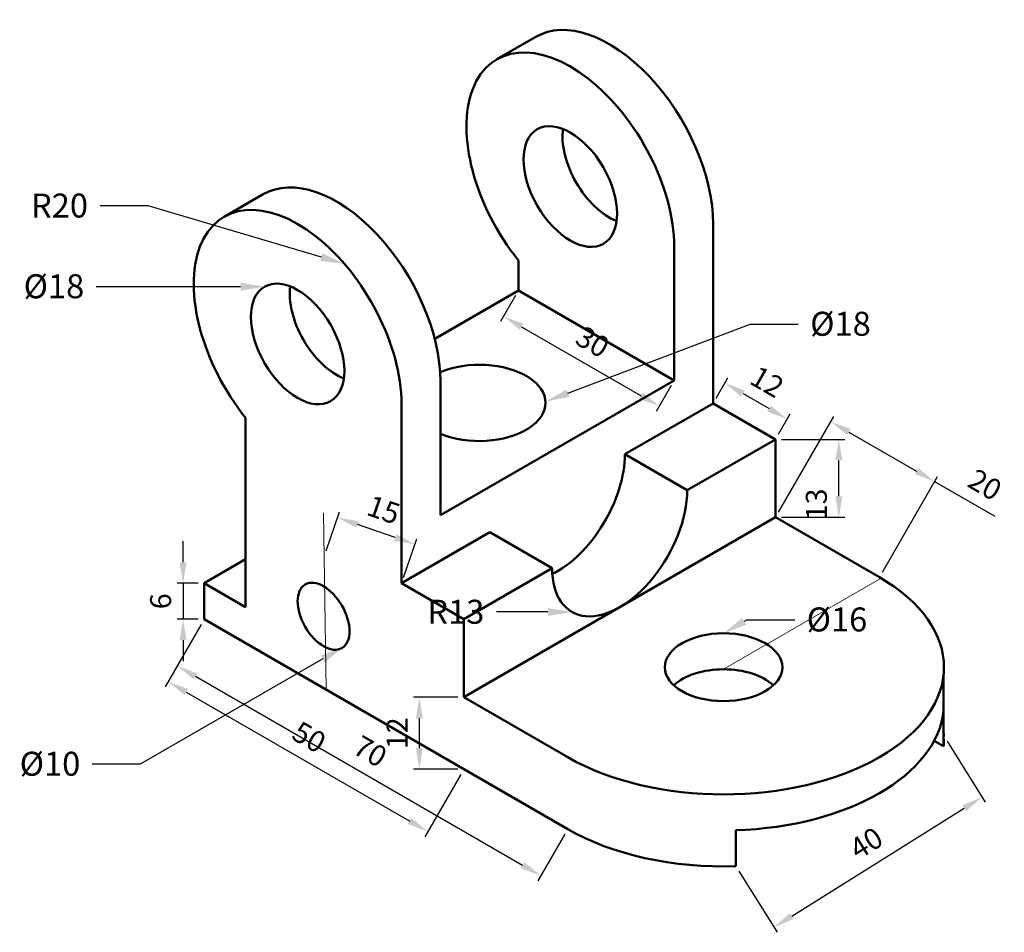
# Model space of a CAD drawing. Units: millimetres. Extents: x 1541 to 1705, y 1721 to 1873.
import ezdxf
from ezdxf import colors
from ezdxf.entities.mleader import LeaderData, LeaderLine
from ezdxf.math import Vec2, Vec3

# ---------------------------------------------------------------- set-up
doc = ezdxf.new("R2010")
doc.units = ezdxf.units.MM
doc.linetypes.add('CENTER', pattern=[50.8, 31.75, -6.35, 6.35, -6.35])
for name, color, linetype, lineweight in [('M-CNTR', 4, 'CENTER', 18), ('M-DIMS', 3, 'Continuous', 25), ('M-OUTL', 7, 'Continuous', 50)]:
    doc.layers.add(name, color=color, linetype=linetype, lineweight=lineweight)
doc.styles.get("Standard").update_dxf_attribs({"font": 'arial.ttf'})
doc.dimstyles.new('AM_ISO$0', dxfattribs={"dimtxt": 3.5, "dimasz": 3.5, "dimexe": 1, "dimexo": 1, "dimgap": 1.5, "dimtad": 1, "dimdsep": 46, "dimtxsty": 'Standard', "dimcen": 0, "dimclrd": 256, "dimclre": 256, "dimclrt": 2, "dimadec": 0, "dimazin": 2, "dimtp": 0.1, "dimtm": 0.1, "dimtfac": 0.71, "dimtdec": 3, "dimtmove": 0, "dimatfit": 3, "dimfxl": 1, "dimlwd": -1, "dimlwe": -1, "dimarcsym": 1})

# ---------------------------------------------------------------- blocks, each defined once
blk = doc.blocks.new('*D3')
at = {"layer": 'Defpoints', "color": 0, "transparency": 16777216}
for p in [(1656.46, 1808.91), (1668.8, 1806.29), (1666.85, 1802.91)]:
    blk.add_point(p, dxfattribs=at)
at = {"layer": 'M-DIMS', "color": 0, "linetype": 'ByBlock', "transparency": 16777216}
for p, q in [((1656.96, 1809.78), (1658.91, 1813.16)), ((1661.44, 1810.54), (1665.77, 1808.04)), ((1667.35, 1803.78), (1669.3, 1807.16))]:
    blk.add_line(p, q, dxfattribs=at)
at = {"layer": 'M-DIMS', "color": 0, "transparency": 16777216}
for points in [[(1661.73, 1811.05), (1661.15, 1810.04), (1658.41, 1812.29)], [(1666.06, 1808.55), (1665.48, 1807.54), (1668.8, 1806.29)]]:
    blk.add_solid(points, dxfattribs=at)
at = {"layer": 'M-DIMS', "color": 0, "transparency": 16777216, "insert": (1665.23, 1812.12), "char_height": 3.5, "attachment_point": 5, "rotation": 330}
blk.add_mtext('12', dxfattribs=at)
blk = doc.blocks.new('*D4')
at = {"layer": 'Defpoints', "color": 0, "transparency": 16777216}
for p in [(1571.59, 1778.91), (1568.08, 1772.91), (1571.59, 1772.91)]:
    blk.add_point(p, dxfattribs=at)
at = {"layer": 'M-DIMS', "color": 0, "linetype": 'ByBlock', "transparency": 16777216}
for p, q in [((1568.08, 1782.41), (1568.08, 1785.91)), ((1570.59, 1778.91), (1567.08, 1778.91)), ((1568.08, 1778.91), (1568.08, 1772.91)), ((1570.59, 1772.91), (1567.08, 1772.91)), ((1568.08, 1769.41), (1568.08, 1765.91))]:
    blk.add_line(p, q, dxfattribs=at)
at = {"layer": 'M-DIMS', "color": 0, "transparency": 16777216}
for points in [[(1567.5, 1782.41), (1568.66, 1782.41), (1568.08, 1778.91)], [(1567.5, 1769.41), (1568.66, 1769.41), (1568.08, 1772.91)]]:
    blk.add_solid(points, dxfattribs=at)
at = {"layer": 'M-DIMS', "color": 0, "transparency": 16777216, "insert": (1564.79, 1775.91), "char_height": 3.5, "attachment_point": 5, "rotation": 90}
blk.add_mtext('6', dxfattribs=at)
blk = doc.blocks.new('*D5')
at = {"layer": 'Defpoints', "color": 0, "transparency": 16777216}
for p in [(1607.47, 1759.91), (1614.89, 1759.91), (1614.89, 1747.91)]:
    blk.add_point(p, dxfattribs=at)
at = {"layer": 'M-DIMS', "color": 0, "linetype": 'ByBlock', "transparency": 16777216}
for p, q in [((1613.89, 1759.91), (1606.47, 1759.91)), ((1607.47, 1751.41), (1607.47, 1756.41)), ((1613.89, 1747.91), (1606.47, 1747.91))]:
    blk.add_line(p, q, dxfattribs=at)
at = {"layer": 'M-DIMS', "color": 0, "transparency": 16777216}
for points in [[(1606.89, 1756.41), (1608.06, 1756.41), (1607.47, 1759.91)], [(1606.89, 1751.41), (1608.06, 1751.41), (1607.47, 1747.91)]]:
    blk.add_solid(points, dxfattribs=at)
at = {"layer": 'M-DIMS', "color": 0, "transparency": 16777216, "insert": (1604.21, 1753.91), "char_height": 3.5, "attachment_point": 5, "rotation": 90}
blk.add_mtext('12', dxfattribs=at)
blk = doc.blocks.new('*D6')
at = {"layer": 'Defpoints', "color": 0, "transparency": 16777216}
for p in [(1694.92, 1753.43), (1701.28, 1743.26), (1660.23, 1731.73)]:
    blk.add_point(p, dxfattribs=at)
at = {"layer": 'M-DIMS', "color": 0, "linetype": 'ByBlock', "transparency": 16777216}
for p, q in [((1695.45, 1752.58), (1701.81, 1742.41)), ((1669.56, 1723.42), (1698.32, 1741.4)), ((1660.76, 1730.89), (1667.13, 1720.71))]:
    blk.add_line(p, q, dxfattribs=at)
at = {"layer": 'M-DIMS', "color": 0, "transparency": 16777216}
for points in [[(1698.01, 1741.9), (1698.63, 1740.91), (1701.28, 1743.26)], [(1669.25, 1723.91), (1669.87, 1722.92), (1666.6, 1721.56)]]:
    blk.add_solid(points, dxfattribs=at)
at = {"layer": 'M-DIMS', "color": 0, "transparency": 16777216, "insert": (1682.2, 1735.2), "char_height": 3.5, "attachment_point": 5, "rotation": 32.027}
blk.add_mtext('40', dxfattribs=at)
blk = doc.blocks.new('*D7')
at = {"layer": 'Defpoints', "color": 0, "transparency": 16777216}
for p in [(1666.85, 1802.91), (1677.4, 1802.91), (1666.85, 1789.91)]:
    blk.add_point(p, dxfattribs=at)
at = {"layer": 'M-DIMS', "color": 0, "linetype": 'ByBlock', "transparency": 16777216}
for p, q in [((1667.85, 1802.91), (1678.4, 1802.91)), ((1677.4, 1793.41), (1677.4, 1799.41)), ((1667.85, 1789.91), (1678.4, 1789.91))]:
    blk.add_line(p, q, dxfattribs=at)
at = {"layer": 'M-DIMS', "color": 0, "transparency": 16777216}
for points in [[(1676.82, 1799.41), (1677.99, 1799.41), (1677.4, 1802.91)], [(1676.82, 1793.41), (1677.99, 1793.41), (1677.4, 1789.91)]]:
    blk.add_solid(points, dxfattribs=at)
at = {"layer": 'M-DIMS', "color": 0, "transparency": 16777216, "insert": (1674.11, 1792.06), "char_height": 3.5, "attachment_point": 5, "rotation": 90}
blk.add_mtext('13', dxfattribs=at)
blk = doc.blocks.new('*D8')
at = {"layer": 'Defpoints', "color": 0, "transparency": 16777216}
for p in [(1693.38, 1795.87), (1666.85, 1789.91), (1684.17, 1779.91)]:
    blk.add_point(p, dxfattribs=at)
at = {"layer": 'M-DIMS', "color": 0, "linetype": 'ByBlock', "transparency": 16777216}
for p, q in [((1667.35, 1790.78), (1676.56, 1806.74)), ((1679.09, 1804.12), (1690.35, 1797.62)), ((1684.67, 1780.78), (1693.88, 1796.74)), ((1693.38, 1795.87), (1703.4, 1790.09))]:
    blk.add_line(p, q, dxfattribs=at)
at = {"layer": 'M-DIMS', "color": 0, "transparency": 16777216}
for points in [[(1679.39, 1804.63), (1678.8, 1803.62), (1676.06, 1805.87)], [(1690.64, 1798.13), (1690.06, 1797.12), (1693.38, 1795.87)]]:
    blk.add_solid(points, dxfattribs=at)
at = {"layer": 'M-DIMS', "color": 0, "transparency": 16777216, "insert": (1701.55, 1794.96), "char_height": 3.5, "attachment_point": 5, "rotation": 330}
blk.add_mtext('20', dxfattribs=at)
blk = doc.blocks.new('*D9')
at = {"layer": 'Defpoints', "color": 0, "transparency": 16777216}
for p in [(1571.59, 1772.91), (1614.89, 1747.91), (1608.89, 1737.52)]:
    blk.add_point(p, dxfattribs=at)
at = {"layer": 'M-DIMS', "color": 0, "linetype": 'ByBlock', "transparency": 16777216}
for p, q in [((1571.09, 1772.05), (1565.09, 1761.66)), ((1568.62, 1760.77), (1605.86, 1739.27)), ((1614.39, 1747.05), (1608.39, 1736.66))]:
    blk.add_line(p, q, dxfattribs=at)
at = {"layer": 'M-DIMS', "color": 0, "transparency": 16777216}
for points in [[(1568.91, 1761.28), (1568.33, 1760.27), (1565.59, 1762.52)], [(1606.15, 1739.78), (1605.56, 1738.77), (1608.89, 1737.52)]]:
    blk.add_solid(points, dxfattribs=at)
at = {"layer": 'M-DIMS', "color": 0, "transparency": 16777216, "insert": (1588.88, 1752.87), "char_height": 3.5, "attachment_point": 5, "rotation": 330}
blk.add_mtext('50', dxfattribs=at)
blk = doc.blocks.new('*D10')
at = {"layer": 'Defpoints', "color": 0, "transparency": 16777216}
for p in [(1623.98, 1827.74), (1649.96, 1812.74), (1647.47, 1808.44)]:
    blk.add_point(p, dxfattribs=at)
at = {"layer": 'M-DIMS', "color": 0, "linetype": 'ByBlock', "transparency": 16777216}
for p, q in [((1623.48, 1826.88), (1620.99, 1822.57)), ((1624.52, 1821.69), (1644.44, 1810.19)), ((1649.46, 1811.88), (1646.97, 1807.57))]:
    blk.add_line(p, q, dxfattribs=at)
at = {"layer": 'M-DIMS', "color": 0, "transparency": 16777216}
for points in [[(1624.82, 1822.19), (1624.23, 1821.18), (1621.49, 1823.44)], [(1644.73, 1810.69), (1644.15, 1809.68), (1647.47, 1808.44)]]:
    blk.add_solid(points, dxfattribs=at)
at = {"layer": 'M-DIMS', "color": 0, "transparency": 16777216, "insert": (1636.13, 1818.78), "char_height": 3.5, "attachment_point": 5, "rotation": 330}
blk.add_mtext('30', dxfattribs=at)
blk = doc.blocks.new('*D11')
at = {"layer": 'Defpoints', "color": 0, "transparency": 16777216}
for p in [(1593.85, 1789.85), (1591.61, 1783.36), (1604.5, 1778.91)]:
    blk.add_point(p, dxfattribs=at)
at = {"layer": 'M-DIMS', "color": 0, "linetype": 'ByBlock', "transparency": 16777216}
for p, q in [((1591.94, 1784.31), (1594.18, 1790.8)), ((1603.43, 1786.55), (1597.16, 1788.71)), ((1604.82, 1779.86), (1607.06, 1786.35))]:
    blk.add_line(p, q, dxfattribs=at)
at = {"layer": 'M-DIMS', "color": 0, "transparency": 16777216}
for points in [[(1597.35, 1789.26), (1596.97, 1788.16), (1593.85, 1789.85)], [(1603.62, 1787.1), (1603.24, 1786), (1606.74, 1785.41)]]:
    blk.add_solid(points, dxfattribs=at)
at = {"layer": 'M-DIMS', "color": 0, "transparency": 16777216, "insert": (1601.37, 1790.74), "char_height": 3.5, "attachment_point": 5, "rotation": 340.9546}
blk.add_mtext('15', dxfattribs=at)
blk = doc.blocks.new('*D12')
at = {"layer": 'Defpoints', "color": 0, "transparency": 16777216}
for p in [(1571.59, 1772.91), (1632.21, 1737.91), (1627.72, 1730.15)]:
    blk.add_point(p, dxfattribs=at)
at = {"layer": 'M-DIMS', "linetype": 'ByBlock', "transparency": 16777216}
for p, q in [((1571.09, 1772.05), (1566.6, 1764.28)), ((1570.13, 1763.4), (1624.69, 1731.9)), ((1631.71, 1737.05), (1627.22, 1729.28))]:
    blk.add_line(p, q, dxfattribs=at)
at = {"layer": 'M-DIMS', "transparency": 16777216}
for points in [[(1570.43, 1763.9), (1569.84, 1762.89), (1567.1, 1765.15)], [(1624.99, 1732.4), (1624.4, 1731.39), (1627.72, 1730.15)]]:
    blk.add_solid(points, dxfattribs=at)
at = {"layer": 'M-DIMS', "color": 2, "transparency": 16777216, "insert": (1599.06, 1750.5), "char_height": 3.5, "attachment_point": 5, "rotation": 330}
blk.add_mtext('70', dxfattribs=at)

msp = doc.modelspace()

# ---------------------------------------------------------------- linework, layer by layer
at = {"layer": 'M-CNTR'}
for p, q in [((1591.505, 1790.666), (1591.942, 1761.162)), ((1658.189, 1764.571), (1684.467, 1779.743))]:
    msp.add_line(p, q, dxfattribs=at)
at = {"layer": 'M-OUTL'}
for p, q in [((1626.889, 1870.028), (1620.394, 1866.278)), ((1581.422, 1843.778), (1574.927, 1840.028)), ((1656.457, 1808.914), (1656.457, 1838.815)), ((1649.961, 1812.744), (1649.961, 1835.065)), ((1623.981, 1827.744), (1623.981, 1832.744)), ((1623.981, 1827.744), (1610.029, 1819.69)), ((1649.961, 1812.744), (1623.981, 1827.744)), ((1610.99, 1790.244), (1649.961, 1812.744)), ((1610.99, 1790.244), (1610.99, 1812.565)), ((1604.495, 1778.914), (1604.495, 1808.815)), ((1641.734, 1800.414), (1656.457, 1808.914)), ((1656.457, 1808.914), (1666.849, 1802.914)), ((1578.514, 1806.494), (1578.514, 1782.914)), ((1652.127, 1794.414), (1666.849, 1802.914)), ((1666.849, 1802.914), (1666.849, 1789.914)), ((1666.849, 1789.914), (1666.849, 1801.914)), ((1641.734, 1800.414), (1652.127, 1794.414)), ((1614.887, 1759.914), (1666.849, 1789.914)), ((1666.849, 1789.914), (1684.169, 1779.914)), ((1604.495, 1778.914), (1619.218, 1787.414)), ((1619.218, 1787.414), (1629.61, 1781.414)), ((1571.586, 1778.914), (1578.514, 1782.914)), ((1578.514, 1782.914), (1578.514, 1774.914)), ((1614.887, 1772.914), (1629.61, 1781.414)), ((1571.586, 1772.914), (1571.586, 1778.914)), ((1571.586, 1778.914), (1578.514, 1774.914)), ((1614.887, 1772.914), (1604.495, 1778.914)), ((1632.208, 1737.914), (1571.586, 1772.914)), ((1614.887, 1759.914), (1614.887, 1772.914)), ((1614.887, 1771.914), (1614.887, 1759.914)), ((1614.887, 1759.914), (1614.887, 1765.914)), ((1694.874, 1763.734), (1694.874, 1754.52)), ((1632.208, 1749.914), (1614.887, 1759.914)), ((1694.869, 1757.734), (1694.869, 1751.734)), ((1694.874, 1754.52), (1694.92, 1753.432)), ((1694.869, 1751.734), (1693.286, 1752.648)), ((1660.233, 1737.734), (1660.233, 1731.734))]:
    msp.add_line(p, q, dxfattribs=at)
for centre, major_axis, start_param, end_param in [((1639.136, 1848.815), (12.247, -21.213), 7.0685835, 9.424778), ((1632.641, 1845.065), (12.247, -21.213), 7.0685835, 11.2573737), ((1639.131, 1848.914), (5.511, -9.546), 3.7717299, 5.6530481), ((1593.67, 1822.565), (12.247, -21.213), 7.0685835, 9.424778), ((1587.175, 1818.815), (12.247, -21.213), 7.0685835, 11.2573737), ((1593.664, 1822.664), (5.511, -9.546), 3.7717299, 5.6530481), ((1617.486, 1808.994), (-11.023, 0), 0.9406591, 5.3481704), ((1630.476, 1793.914), (-7.961, -13.789), 6.9943465, 8.6393798), ((1640.868, 1787.914), (-7.961, -13.789), 5.4977871, 8.6393798), ((1658.189, 1764.914), (-36.742, 0), 7.0685835, 10.2101761), ((1658.189, 1758.914), (-9.798, 0), 3.7005825, 5.7241954), ((1658.189, 1758.914), (-36.742, 0), 7.9096521, 9.3691075), ((1658.183, 1752.914), (36.742, 0), 6.2275148, 6.2831853), ((1658.189, 1752.914), (-36.742, 0), 7.0685835, 7.9096521)]:
    msp.add_ellipse(centre, major_axis=major_axis, ratio=0.5773503, start_param=start_param, end_param=end_param, dxfattribs=at)
for centre, major_axis in [((1632.641, 1845.065), (5.511, -9.546)), ((1587.175, 1818.815), (5.511, -9.546)), ((1591.505, 1773.414), (3.062, -5.303)), ((1658.189, 1764.914), (-9.798, 0))]:
    msp.add_ellipse(centre, major_axis=major_axis, ratio=0.5773503, dxfattribs=at)

# ---------------------------------------------------------------- dimensions: what is measured, and where the dimension line sits
at = {"layer": 'M-DIMS'}
for p1, p2, distance, override, picture, middle in [((1623.981, 1827.744), (1649.961, 1812.744), -4.974, {"dimpost": '', "dimclrd": 0, "dimclre": 0, "dimclrt": 0}, '*D10', (1636.128, 1818.784)), ((1656.457, 1808.914), (1666.849, 1802.914), 3.903, {"dimpost": '', "dimclrd": 0, "dimclre": 0, "dimclrt": 0}, '*D3', (1665.233, 1812.115)), ((1571.586, 1778.914), (1571.586, 1772.914), -3.507, {"dimpost": '', "dimclrd": 0, "dimclre": 0, "dimclrt": 0}, '*D4', (1564.792, 1775.914)), ((1571.586, 1772.914), (1614.887, 1747.914), -12, {"dimpost": '', "dimclrd": 0, "dimclre": 0, "dimclrt": 0}, '*D9', (1588.88, 1752.869)), ((1614.887, 1747.914), (1614.887, 1759.914), 7.415, {"dimclrd": 0, "dimclre": 0, "dimclrt": 0}, '*D5', (1604.215, 1753.914))]:
    dim = msp.add_aligned_dim(p1=p1, p2=p2, distance=distance, dimstyle='AM_ISO$0', override=override, dxfattribs=at)
    dim.commit()
    dim.dimension.update_dxf_attribs({"geometry": picture, "text_midpoint": middle})
for base, p2, angle, picture, middle in [((1693.384, 1795.875), (1684.169, 1779.914), 330, '*D8', (1699.906, 1792.109)), ((1677.402, 1802.914), (1666.849, 1802.914), 90, '*D7', (1677.402, 1792.063))]:
    dim = msp.add_linear_dim(base=base, p1=(1666.849, 1789.914), p2=p2, angle=angle, dimstyle='AM_ISO$0', override={"dimclrd": 0, "dimclre": 0, "dimclrt": 0}, dxfattribs=at)
    dim.commit()
    dim.dimension.update_dxf_attribs({"geometry": picture, "text_midpoint": middle, "dimtype": 161})
for p1, p2, distance, text, picture, middle in [((1604.495, 1778.914), (1591.613, 1783.361), -6.869, '15', '*D11', (1601.368, 1790.738)), ((1660.233, 1731.734), (1694.92, 1753.432), -12, '40', '*D6', (1682.197, 1735.196))]:
    dim = msp.add_aligned_dim(p1=p1, p2=p2, distance=distance, text=text, dimstyle='AM_ISO$0', override={"dimpost": '', "dimclrd": 0, "dimclre": 0, "dimclrt": 0}, dxfattribs=at)
    dim.commit()
    dim.dimension.update_dxf_attribs({"geometry": picture, "text_midpoint": middle})
dim = msp.add_linear_dim(base=(1627.724, 1730.149), p1=(1571.586, 1772.914), p2=(1632.208, 1737.914), angle=330, dimstyle='AM_ISO$0', override={"dimrnd": 0}, dxfattribs=at)
dim.commit()
dim.dimension.update_dxf_attribs({"geometry": '*D12', "text_midpoint": (1599.057, 1750.495)})

# ---------------------------------------------------------------- leaders
ml = msp.add_multileader_mtext('Standard', dxfattribs=at)
ml.set_content('{\\C2;R20}', color=256)
ml.set_leader_properties()
ml.build(insert=Vec2(0, 0))
ctx = ml.context
ctx.base_point, ctx.plane_origin = Vec3(1540.69, 1841.863), Vec3(1594.984, 1832.158)
ctx.text_align_type = 2
notes = []
notes.append((ctx, [(0, (1, 1, 0), (1562.235, 1841.863), (-1, 0), 8, [(0, [(1594.984, 1832.158)], 0, [])])]))
ctx.mtext.insert, ctx.mtext.alignment, ctx.mtext.flow_direction = Vec3(1552.235, 1843.897), 3, 5
ml = msp.add_multileader_mtext('Standard', dxfattribs=at)
ml.set_content('{\\C2;%%C18}', color=256)
ml.set_leader_properties()
ml.build(insert=Vec2(0, 0))
ctx = ml.context
ctx.base_point, ctx.plane_origin = Vec3(1539.518, 1828.361), Vec3(1581.663, 1828.361)
ctx.text_align_type = 2
notes.append((ctx, [(0, (1, 1, 0), (1561.608, 1828.361), (-1, 0), 8, [(0, [(1581.663, 1828.361)], 0, [])])]))
ctx.mtext.insert, ctx.mtext.alignment, ctx.mtext.flow_direction = Vec3(1551.608, 1830.441), 3, 5
ml = msp.add_multileader_mtext('Standard', dxfattribs=at)
ml.set_content('{\\C2;%%C18}', color=256)
ml.set_leader_properties()
ml.build(insert=Vec2(0, 0))
ctx = ml.context
ctx.base_point, ctx.plane_origin = Vec3(1670.629, 1822.101), Vec3(1628.502, 1809.203)
notes.append((ctx, [(0, (1, 1, 0), (1662.629, 1822.101), (1, 0), 8, [(0, [(1628.502, 1809.203)], 0, [])])]))
ctx.mtext.insert, ctx.mtext.flow_direction = Vec3(1672.629, 1824.182), 5
ml = msp.add_multileader_mtext('Standard', dxfattribs=at)
ml.set_content('{\\C2;R13}', color=256)
ml.set_leader_properties()
ml.build(insert=Vec2(0, 0))
ctx = ml.context
ctx.base_point, ctx.plane_origin = Vec3(1606.751, 1774.126), Vec3(1632.907, 1774.126)
ctx.text_align_type = 2
notes.append((ctx, [(0, (1, 1, 0), (1628.309, 1774.126), (-1, 0), 8, [(0, [(1632.907, 1774.126)], 0, [])])]))
ctx.mtext.insert, ctx.mtext.alignment, ctx.mtext.flow_direction = Vec3(1618.309, 1776.161), 3, 5
ml = msp.add_multileader_mtext('Standard', dxfattribs=at)
ml.set_content('{\\C2;%%C16}', color=256)
ml.set_leader_properties()
ml.build(insert=Vec2(0, 0))
ctx = ml.context
ctx.base_point, ctx.plane_origin = Vec3(1670.044, 1772.797), Vec3(1658.189, 1770.571)
notes.append((ctx, [(0, (1, 1, 0), (1662.044, 1772.797), (1, 0), 8, [(0, [(1658.189, 1770.571)], 0, [])])]))
ctx.mtext.insert, ctx.mtext.flow_direction = Vec3(1672.044, 1774.878), 5
ml = msp.add_multileader_mtext('Standard', dxfattribs=at)
ml.set_content('{\\C2;%%C10}', color=256)
ml.set_leader_properties()
ml.build(insert=Vec2(0, 0))
ctx = ml.context
ctx.base_point, ctx.plane_origin = Vec3(1538.88, 1748.735), Vec3(1594.851, 1768.309)
ctx.text_align_type = 2
notes.append((ctx, [(0, (1, 1, 0), (1560.948, 1748.735), (-1, 0), 8, [(0, [(1594.851, 1768.309)], 0, [])])]))
ctx.mtext.insert, ctx.mtext.alignment, ctx.mtext.flow_direction = Vec3(1550.948, 1750.816), 3, 5
for ctx, leaders in notes:
    for number, flags, end, landing, length, lines in leaders:
        leader = LeaderData()
        leader.index, (leader.has_last_leader_line, leader.has_dogleg_vector, leader.attachment_direction) = number, flags
        leader.last_leader_point, leader.dogleg_vector, leader.dogleg_length = Vec3(end), Vec3(landing), length
        for number, points, colour, breaks in lines:
            line = LeaderLine()
            line.index, line.vertices, line.color, line.breaks = number, Vec3.list(points), colors.encode_raw_color(colour), breaks
            leader.lines.append(line)
        ctx.leaders.append(leader)

doc.saveas('drawing.dxf')
